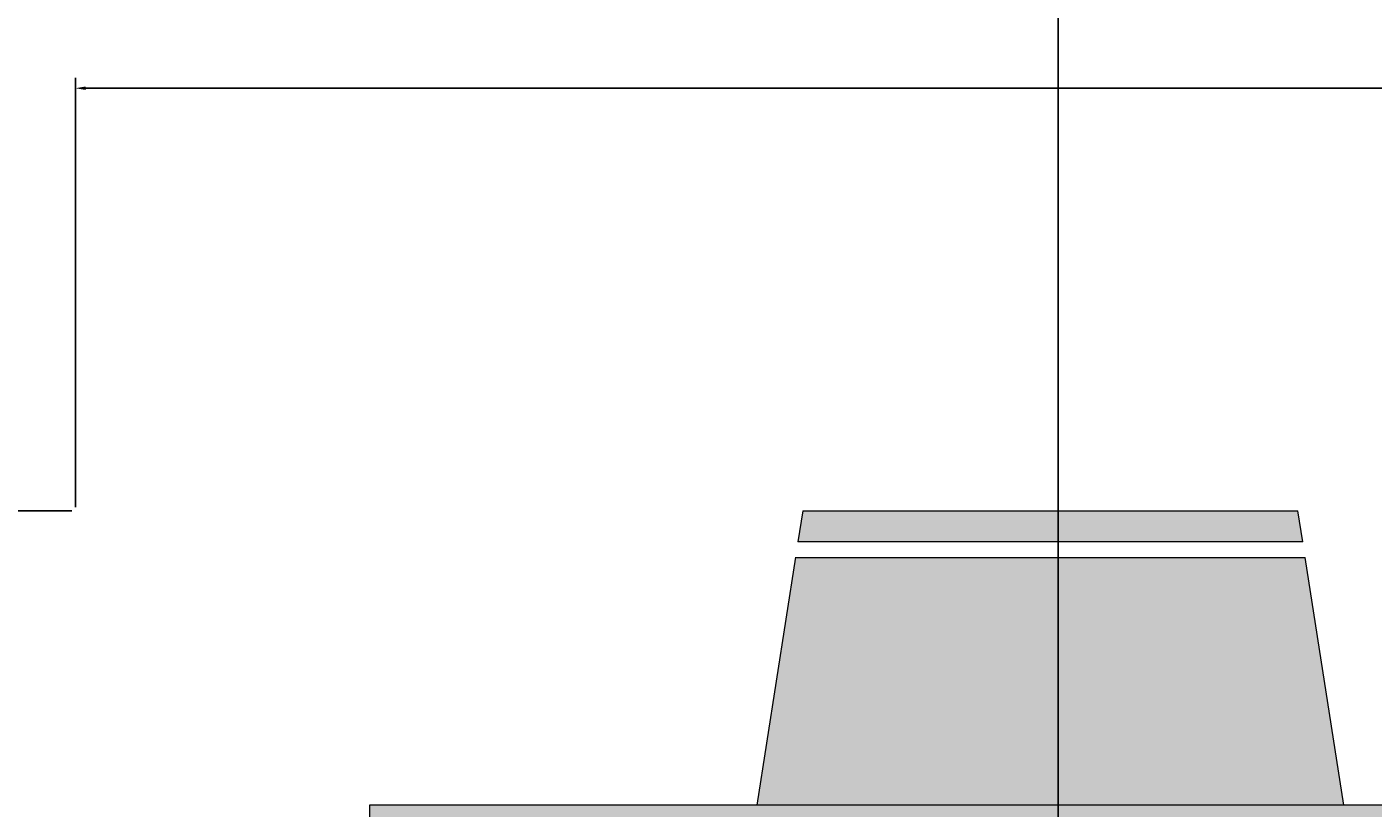
# Model space of a CAD drawing. Units: inches. Extents: x 2549 to 3108, y 1683 to 2362.
# Tile 10 of 30: x 2711 to 2734, y 2041 to 2055. Entities that reach past the tile are written whole.
import ezdxf

# ---------------------------------------------------------------- set-up
doc = ezdxf.new("R2010")
doc.units = ezdxf.units.IN
for name, color, linetype, lineweight in [('A-ANNO-DIMS', 2, 'Continuous', 18), ('A-FURN', 8, 'Continuous', 18), ('A-FURN-PATT', 9, 'Continuous', 13)]:
    doc.layers.add(name, color=color, linetype=linetype, lineweight=lineweight)
doc.layers.add('C-PKNG-VEHI-PATT', color=251, linetype='Continuous', lineweight=13, true_color=0x636466)
doc.layers.add('C-PVMT-PATT', color=9, linetype='Continuous', lineweight=13, true_color=0xc7c8ca)
doc.styles.get("Standard").update_dxf_attribs({"font": 'arial.ttf'})
doc.dimstyles.get("Standard").update_dxf_attribs({"dimtxt": 0.18, "dimasz": 0.18, "dimexe": 0.18, "dimexo": 0.0625, "dimgap": 0.09, "dimtad": 0, "dimtih": 1, "dimtoh": 1, "dimdec": 4, "dimzin": 0, "dimdsep": 46, "dimtxsty": 'Standard', "dimcen": 0.09, "dimadec": 0, "dimazin": 0, "dimtfac": 1, "dimtdec": 4, "dimtofl": 0, "dimtmove": 0, "dimatfit": 3, "dimfxl": 1, "dimtolj": 1, "dimtzin": 0, "dimarcsym": 0})

# ---------------------------------------------------------------- blocks, each defined once
blk = doc.blocks.new('Dining Set - 36 x 72 in.')
for p, q in [((-22, 27.5), (-22.1562, 26.50042)), ((-22, 27.5), (-6, 27.5)), ((-5.8437, 26.49966), (-6, 27.5)), ((-5.8416, 26.5), (-22.1534, 26.5)), ((-22.2343, 26.00059), (-23.4847, 17.99762)), ((-22.2304, 26), (-5.7608, 26)), ((-4.5152, 17.99762), (-5.7655, 25.99926)), ((36, 18), (-36, 18)), ((-36, 18), (-36, -18))]:
    blk.add_line(p, q)
blk = doc.blocks.new('*D20')
at = {"layer": 'A-ANNO-DIMS', "color": 0, "lineweight": -2, "transparency": 16777216}
for p, q in [((2711.514, 2046.346), (2711.514, 2053.826)), ((2711.694, 2053.646), (2735.087, 2053.646)), ((2760.417, 2053.646), (2737.025, 2053.646)), ((2760.597, 2046.346), (2760.597, 2053.826))]:
    blk.add_line(p, q, dxfattribs=at)
at = {"layer": 'A-ANNO-DIMS', "color": 0, "transparency": 16777216}
for points in [[(2711.694, 2053.676), (2711.694, 2053.616), (2711.514, 2053.646)], [(2760.417, 2053.676), (2760.417, 2053.616), (2760.597, 2053.646)]]:
    blk.add_solid(points, dxfattribs=at)
at = {"layer": 'Defpoints', "color": 0, "transparency": 16777216}
for p in [(2760.597, 2053.646), (2711.514, 2046.283), (2760.597, 2046.283)]:
    blk.add_point(p, dxfattribs=at)
at = {"layer": 'A-ANNO-DIMS', "color": 0, "transparency": 16777216, "insert": (2736.056, 2053.646), "char_height": 0.18, "attachment_point": 5}
blk.add_mtext('\\A1;DINING SET 49', dxfattribs=at)
blk = doc.blocks.new('*D21')
at = {"layer": 'A-ANNO-DIMS', "color": 0, "lineweight": -2, "transparency": 16777216}
for p, q in [((2711.452, 2046.283), (2703.972, 2046.283)), ((2704.152, 2046.103), (2704.152, 2031.633)), ((2704.152, 2016.798), (2704.152, 2031.269)), ((2711.452, 2016.618), (2703.972, 2016.618))]:
    blk.add_line(p, q, dxfattribs=at)
at = {"layer": 'A-ANNO-DIMS', "color": 0, "transparency": 16777216}
for points in [[(2704.122, 2046.103), (2704.182, 2046.103), (2704.152, 2046.283)], [(2704.122, 2016.798), (2704.182, 2016.798), (2704.152, 2016.618)]]:
    blk.add_solid(points, dxfattribs=at)
at = {"layer": 'Defpoints', "color": 0, "transparency": 16777216}
for p in [(2704.152, 2046.283), (2711.514, 2046.283), (2711.514, 2016.618)]:
    blk.add_point(p, dxfattribs=at)
at = {"layer": 'A-ANNO-DIMS', "color": 0, "transparency": 16777216, "insert": (2704.152, 2031.451), "char_height": 0.18, "attachment_point": 5}
blk.add_mtext('\\A1;30', dxfattribs=at)
blk = doc.blocks.new('*D42')
at = {"layer": 'A-ANNO-DIMS', "color": 0, "lineweight": -2, "transparency": 16777216}
for p, q in [((2638.643, 2080.461), (2638.643, 1683.444)), ((2728.643, 2080.461), (2728.643, 1683.444)), ((2638.823, 1683.624), (2683.424, 1683.624)), ((2728.463, 1683.624), (2683.861, 1683.624))]:
    blk.add_line(p, q, dxfattribs=at)
at = {"layer": 'A-ANNO-DIMS', "color": 0, "transparency": 16777216}
for points in [[(2638.823, 1683.654), (2638.823, 1683.594), (2638.643, 1683.624)], [(2728.463, 1683.654), (2728.463, 1683.594), (2728.643, 1683.624)]]:
    blk.add_solid(points, dxfattribs=at)
at = {"layer": 'Defpoints', "color": 0, "transparency": 16777216}
for p in [(2638.643, 2080.524), (2728.643, 2080.524), (2728.643, 1683.624)]:
    blk.add_point(p, dxfattribs=at)
at = {"layer": 'A-ANNO-DIMS', "color": 0, "transparency": 16777216, "insert": (2683.643, 1683.624), "char_height": 0.18, "attachment_point": 5}
blk.add_mtext('\\A1;90', dxfattribs=at)
blk = doc.blocks.new('*D59')
at = {"layer": 'A-ANNO-DIMS', "color": 0, "lineweight": -2, "transparency": 16777216}
for p, q in [((2680.978, 1761.586), (2680.978, 2362.323)), ((2681.158, 2362.143), (2733.112, 2362.143)), ((2785.978, 2362.143), (2734.023, 2362.143)), ((2786.158, 1761.586), (2786.158, 2362.323))]:
    blk.add_line(p, q, dxfattribs=at)
at = {"layer": 'A-ANNO-DIMS', "color": 0, "transparency": 16777216}
for points in [[(2681.158, 2362.173), (2681.158, 2362.113), (2680.978, 2362.143)], [(2785.978, 2362.173), (2785.978, 2362.113), (2786.158, 2362.143)]]:
    blk.add_solid(points, dxfattribs=at)
at = {"layer": 'Defpoints', "color": 0, "transparency": 16777216}
for p in [(2786.158, 2362.143), (2680.978, 1761.524), (2786.158, 1761.524)]:
    blk.add_point(p, dxfattribs=at)
at = {"layer": 'A-ANNO-DIMS', "color": 0, "transparency": 16777216, "insert": (2733.568, 2362.143), "char_height": 0.18, "attachment_point": 5}
blk.add_mtext('\\A1;105.18', dxfattribs=at)

msp = doc.modelspace()

# ---------------------------------------------------------------- hatches: boundary and pattern name
at = {"layer": 'A-FURN-PATT'}
h = msp.add_hatch(color=256, dxfattribs=at)
h.dxf.hatch_style = 1
h.paths.add_polyline_path([(2732.9458, 2045.4744), (2724.0631, 2045.4744), (2723.389, 2041.1594), (2733.6201, 2041.1594)])
h.paths.add_polyline_path([(2748.0481, 2045.4744), (2739.1654, 2045.4744), (2738.4912, 2041.1594), (2748.7223, 2041.1594)])
h.paths.add_polyline_path([(2747.9217, 2046.2834), (2739.2918, 2046.2834), (2739.2075, 2045.7441), (2748.006, 2045.7441)])
h.paths.add_polyline_path([(2732.8194, 2046.2834), (2724.1896, 2046.2834), (2724.1053, 2045.7441), (2732.9037, 2045.7441)])
h.paths.add_polyline_path([(2759.7877, 2035.8922), (2755.4728, 2036.5664), (2755.4728, 2026.3353), (2759.7877, 2027.0095)])
h.paths.add_polyline_path([(2760.5968, 2035.7658), (2760.0574, 2035.8501), (2760.0574, 2027.0516), (2760.5968, 2027.1359)])
h.paths.add_polyline_path([(2716.6384, 2036.5664), (2712.3235, 2035.8922), (2712.3235, 2027.0095), (2716.6384, 2026.3353)])
h.paths.add_polyline_path([(2733.6201, 2021.7423), (2723.389, 2021.7423), (2724.0631, 2017.4273), (2732.9458, 2017.4273)])
h.paths.add_polyline_path([(2748.7223, 2021.7423), (2738.4912, 2021.7423), (2739.1654, 2017.4273), (2748.0481, 2017.4273)])
h.paths.add_polyline_path([(2748.006, 2017.1576), (2739.2075, 2017.1576), (2739.2918, 2016.6183), (2747.9217, 2016.6183)])
h.paths.add_polyline_path([(2732.9037, 2017.1576), (2724.1053, 2017.1576), (2724.1896, 2016.6183), (2732.8194, 2016.6183)])
h.paths.add_polyline_path([(2712.0538, 2035.85), (2711.5145, 2035.7658), (2711.5145, 2027.1359), (2712.0538, 2027.0516)])
h = msp.add_hatch(color=256, dxfattribs=at)
h.dxf.hatch_style = 1
h.paths.add_polyline_path([(2744.8667, 2037.254), (2744.7754, 2037.3839), (2744.7125, 2037.4849), (2744.6595, 2037.5854), (2744.5963, 2037.7375), (2744.5695, 2037.9287), (2744.6003, 2038.0617), (2744.6406, 2038.148), (2744.7014, 2038.2298), (2744.7817, 2038.3053), (2744.8799, 2038.3724), (2744.9945, 2038.4289), (2745.1238, 2038.4728), (2745.2663, 2038.5019), (2745.4204, 2038.5142), (2745.5844, 2038.5076), (2745.7585, 2038.4805), (2745.9486, 2038.4342), (2746.1624, 2038.3705), (2746.4075, 2038.2913), (2746.6917, 2038.1983), (2747.0224, 2038.0936), (2747.4074, 2037.9788), (2747.8543, 2037.8558), (2748.3724, 2037.7256), (2748.9783, 2037.5851), (2749.69, 2037.4304), (2750.5258, 2037.2575), (2751.5038, 2037.0624), (2752.6422, 2036.8414), (2753.9591, 2036.5902), (2755.4728, 2036.3051), (2755.4728, 2039.002), (2754.0892, 2039.103), (2752.7721, 2039.2035), (2751.5251, 2039.303), (2750.3516, 2039.4009), (2749.255, 2039.4967), (2748.2388, 2039.5898), (2747.3063, 2039.6798), (2746.4609, 2039.7661), (2745.7045, 2039.8482), (2745.0321, 2039.9255), (2744.4371, 2039.9976), (2743.9129, 2040.0639), (2743.4531, 2040.1238), (2743.0509, 2040.1769), (2742.6998, 2040.2227), (2742.3932, 2040.2605), (2742.1251, 2040.29), (2741.8917, 2040.3111), (2741.69, 2040.3237), (2741.5167, 2040.3279), (2741.3687, 2040.3237), (2741.2428, 2040.3111), (2741.1359, 2040.29), (2741.0448, 2040.2605), (2740.9668, 2040.2227), (2740.9015, 2040.1776), (2740.8488, 2040.1262), (2740.8088, 2040.0695), (2740.7814, 2040.0085), (2740.7667, 2039.9445), (2740.7646, 2039.8783), (2740.7751, 2039.811), (2740.7978, 2039.7435), (2740.8306, 2039.6755), (2740.8707, 2039.6064), (2740.9155, 2039.5357), (2740.996, 2039.4111), (2741.0771, 2039.2637), (2741.1346, 2039.0945), (2741.1499, 2038.9139), (2741.1092, 2038.7391), (2741.0289, 2038.6239), (2740.9549, 2038.5525), (2740.8586, 2038.4895), (2740.733, 2038.4359), (2740.5693, 2038.3929), (2740.3593, 2038.3615), (2740.0946, 2038.3427), (2739.7666, 2038.3376), (2739.367, 2038.3473), (2738.8873, 2038.3727), (2738.3203, 2038.4145), (2737.6635, 2038.471), (2736.9156, 2038.5402), (2736.0753, 2038.6199), (2735.1412, 2038.7081), (2734.112, 2038.8025), (2732.9864, 2038.9012), (2731.7632, 2039.002), (2730.4376, 2039.1026), (2728.9922, 2039.2), (2727.4062, 2039.2911), (2725.6588, 2039.3728), (2723.7291, 2039.4418), (2721.5964, 2039.495), (2719.2397, 2039.5292), (2716.6384, 2039.5413), (2716.6384, 2036.8445), (2720.4266, 2036.9215), (2723.5572, 2036.9548), (2726.1183, 2036.9512), (2728.1983, 2036.9175), (2729.8853, 2036.8608), (2731.2677, 2036.7876), (2732.4336, 2036.705), (2733.4711, 2036.6198), (2734.4538, 2036.5375), (2735.3951, 2036.4589), (2736.2938, 2036.3835), (2737.1484, 2036.3108), (2737.9578, 2036.2401), (2738.7205, 2036.171), (2739.4353, 2036.103), (2740.1009, 2036.0355), (2740.7163, 2035.9683), (2741.2828, 2035.9027), (2741.8019, 2035.8403), (2742.2752, 2035.7826), (2742.7042, 2035.7313), (2743.0906, 2035.6878), (2743.4358, 2035.6539), (2743.7416, 2035.6309), (2744.0097, 2035.6203), (2744.243, 2035.6218), (2744.4448, 2035.6349), (2744.6181, 2035.659), (2744.7661, 2035.6937), (2744.892, 2035.7384), (2744.9989, 2035.7926), (2745.09, 2035.8557), (2745.1679, 2035.9271), (2745.2326, 2036.006), (2745.2836, 2036.0911), (2745.3204, 2036.1815), (2745.3424, 2036.2762), (2745.3492, 2036.374), (2745.3401, 2036.4739), (2745.3148, 2036.5748), (2745.2731, 2036.676), (2745.2178, 2036.7771), (2745.152, 2036.8782), (2745.0788, 2036.9794), (2745.0013, 2037.0805)])
h.paths.add_polyline_path([(2755.4728, 2036.3051), (2753.9591, 2036.5902), (2752.6422, 2036.8414), (2751.5038, 2037.0624), (2750.5258, 2037.2575), (2749.69, 2037.4304), (2748.9783, 2037.5851), (2748.3724, 2037.7256), (2747.8543, 2037.8558), (2747.4074, 2037.9788), (2747.0224, 2038.0936), (2746.6917, 2038.1983), (2746.4075, 2038.2913), (2746.1624, 2038.3705), (2745.9486, 2038.4342), (2745.7585, 2038.4805), (2745.5844, 2038.5076), (2745.4204, 2038.5142), (2745.2663, 2038.5019), (2745.1238, 2038.4728), (2744.9945, 2038.4289), (2744.8799, 2038.3724), (2744.7817, 2038.3053), (2744.7014, 2038.2298), (2744.6406, 2038.148), (2744.6003, 2038.0617), (2744.5794, 2037.9717), (2744.5765, 2037.8786), (2744.59, 2037.7828), (2744.6182, 2037.6849), (2744.6595, 2037.5854), (2744.7125, 2037.4849), (2744.7754, 2037.3839), (2744.8465, 2037.2827), (2744.9229, 2037.1816), (2745.0013, 2037.0805), (2745.1278, 2036.9154), (2745.2178, 2036.7771), (2745.2731, 2036.676), (2745.3148, 2036.5748), (2745.3401, 2036.4739), (2745.3492, 2036.374), (2745.3424, 2036.2762), (2745.3204, 2036.1815), (2745.2836, 2036.0911), (2745.2326, 2036.006), (2745.1679, 2035.9271), (2745.09, 2035.8557), (2744.9989, 2035.7926), (2744.892, 2035.7384), (2744.7661, 2035.6937), (2744.6181, 2035.659), (2744.4448, 2035.6349), (2744.243, 2035.6218), (2744.0097, 2035.6203), (2743.7416, 2035.6309), (2743.4358, 2035.6539), (2743.0906, 2035.6878), (2742.7042, 2035.7313), (2742.2752, 2035.7826), (2741.8019, 2035.8403), (2741.2828, 2035.9027), (2740.7163, 2035.9683), (2740.1009, 2036.0355), (2739.4353, 2036.103), (2738.7205, 2036.171), (2737.9578, 2036.2401), (2737.1484, 2036.3108), (2736.2938, 2036.3835), (2735.3951, 2036.4589), (2734.4538, 2036.5375), (2733.4711, 2036.6198), (2732.4336, 2036.705), (2731.2677, 2036.7876), (2729.8853, 2036.8608), (2728.1983, 2036.9175), (2726.1183, 2036.9512), (2723.5572, 2036.9548), (2720.4266, 2036.9215), (2716.6384, 2036.8445), (2716.6384, 2034.4174), (2719.4886, 2034.3283), (2721.9949, 2034.2608), (2724.1925, 2034.2112), (2726.1167, 2034.1758), (2727.8028, 2034.1509), (2729.2861, 2034.1329), (2730.602, 2034.1181), (2731.7856, 2034.1027), (2732.8685, 2034.0839), (2733.8666, 2034.0613), (2734.7919, 2034.0356), (2735.6567, 2034.0072), (2736.473, 2033.9768), (2737.253, 2033.9447), (2738.0088, 2033.9116), (2738.7525, 2033.878), (2739.493, 2033.8445), (2740.2273, 2033.812), (2740.9489, 2033.7816), (2741.6515, 2033.7544), (2742.3289, 2033.7314), (2742.9747, 2033.7137), (2743.5825, 2033.7022), (2744.1461, 2033.6982), (2744.6607, 2033.7024), (2745.1272, 2033.7151), (2745.5485, 2033.7361), (2745.9272, 2033.7656), (2746.2658, 2033.8036), (2746.567, 2033.8499), (2746.8334, 2033.9047), (2747.0677, 2033.9679), (2747.2728, 2034.0393), (2747.4525, 2034.1175), (2747.6113, 2034.201), (2747.7531, 2034.2881), (2747.8824, 2034.3774), (2748.0032, 2034.4672), (2748.1197, 2034.556), (2748.2363, 2034.6421), (2748.3567, 2034.7241), (2748.4828, 2034.8008), (2748.6163, 2034.8712), (2748.7588, 2034.9343), (2748.9118, 2034.9889), (2749.077, 2035.034), (2749.2558, 2035.0686), (2749.4499, 2035.0916), (2749.6603, 2035.1022), (2749.8861, 2035.1007), (2750.1254, 2035.0876), (2750.3769, 2035.0635), (2750.639, 2035.0288), (2750.91, 2034.9841), (2751.1884, 2034.93), (2751.4725, 2034.8668), (2751.7642, 2034.7949), (2752.0786, 2034.7123), (2752.4341, 2034.6172), (2752.849, 2034.5073), (2753.3419, 2034.3805), (2753.9313, 2034.2348), (2754.6354, 2034.068), (2755.4728, 2033.878)])
h.paths.add_polyline_path([(2755.4728, 2033.878), (2754.6354, 2034.068), (2753.9313, 2034.2348), (2753.3419, 2034.3805), (2752.849, 2034.5073), (2752.4341, 2034.6172), (2752.0786, 2034.7123), (2751.7642, 2034.7949), (2751.4725, 2034.8668), (2751.1884, 2034.93), (2750.91, 2034.9841), (2750.639, 2035.0288), (2750.3769, 2035.0635), (2750.1254, 2035.0876), (2749.8861, 2035.1007), (2749.6603, 2035.1022), (2749.4499, 2035.0916), (2749.2558, 2035.0686), (2749.077, 2035.034), (2748.9118, 2034.9889), (2748.7588, 2034.9343), (2748.6163, 2034.8712), (2748.4828, 2034.8008), (2748.3567, 2034.7241), (2748.2363, 2034.6421), (2748.1197, 2034.556), (2748.0032, 2034.4672), (2747.8824, 2034.3774), (2747.7531, 2034.2881), (2747.6113, 2034.201), (2747.4525, 2034.1175), (2747.2728, 2034.0393), (2747.0677, 2033.9679), (2746.8334, 2033.9047), (2746.567, 2033.8499), (2746.2658, 2033.8036), (2745.9272, 2033.7656), (2745.5485, 2033.7361), (2745.1272, 2033.7151), (2744.6607, 2033.7024), (2744.1461, 2033.6982), (2743.5825, 2033.7022), (2742.9747, 2033.7137), (2742.3289, 2033.7314), (2741.6515, 2033.7544), (2740.9489, 2033.7816), (2740.2273, 2033.812), (2739.493, 2033.8445), (2738.7525, 2033.878), (2738.0088, 2033.9116), (2737.253, 2033.9447), (2736.473, 2033.9768), (2735.6567, 2034.0072), (2734.7919, 2034.0356), (2733.8666, 2034.0613), (2732.8685, 2034.0839), (2731.7856, 2034.1027), (2730.602, 2034.1181), (2729.2861, 2034.1329), (2727.8028, 2034.1509), (2726.1167, 2034.1758), (2724.1925, 2034.2112), (2721.9949, 2034.2608), (2719.4886, 2034.3283), (2716.6384, 2034.4174), (2716.6384, 2030.9115), (2719.4477, 2031.0954), (2722.0216, 2031.2447), (2724.3773, 2031.363), (2726.5324, 2031.4537), (2728.5042, 2031.5201), (2730.3101, 2031.5657), (2731.9674, 2031.5939), (2733.4936, 2031.6082), (2734.9046, 2031.6115), (2736.2109, 2031.6057), (2737.4211, 2031.592), (2738.5446, 2031.5716), (2739.59, 2031.5461), (2740.5665, 2031.5165), (2741.4829, 2031.4843), (2742.3482, 2031.4509), (2743.1698, 2031.4174), (2743.9488, 2031.3855), (2744.6845, 2031.3568), (2745.3766, 2031.3329), (2746.0244, 2031.3152), (2746.6274, 2031.3055), (2747.1851, 2031.3052), (2747.697, 2031.316), (2748.1634, 2031.3388), (2748.5882, 2031.3722), (2748.9761, 2031.414), (2749.3319, 2031.4621), (2749.6603, 2031.5144), (2749.9661, 2031.5688), (2750.254, 2031.6233), (2750.5287, 2031.6756), (2750.7946, 2031.7239), (2751.0553, 2031.7669), (2751.314, 2031.8036), (2751.5737, 2031.8329), (2751.8375, 2031.8538), (2752.1088, 2031.8652), (2752.3906, 2031.8661), (2752.6861, 2031.8554), (2752.9965, 2031.8326), (2753.315, 2031.7999), (2753.633, 2031.7598), (2753.9418, 2031.7149), (2754.2327, 2031.6679), (2754.497, 2031.6215), (2754.7259, 2031.5782), (2754.911, 2031.5407), (2755.0467, 2031.5111), (2755.141, 2031.4888), (2755.2053, 2031.4728), (2755.2509, 2031.4621), (2755.2891, 2031.4556), (2755.3313, 2031.4523), (2755.3888, 2031.451), (2755.4728, 2031.4509)])
h.paths.add_polyline_path([(2743.9488, 2031.3855), (2743.1698, 2031.4174), (2742.3482, 2031.4509), (2741.4829, 2031.4843), (2740.5665, 2031.5165), (2739.59, 2031.5461), (2738.5446, 2031.5716), (2737.4211, 2031.592), (2736.2109, 2031.6057), (2734.9046, 2031.6115), (2733.4936, 2031.6082), (2731.9674, 2031.5939), (2730.3101, 2031.5657), (2728.5042, 2031.5201), (2726.5324, 2031.4537), (2724.3773, 2031.363), (2722.0216, 2031.2447), (2719.4477, 2031.0954), (2716.6384, 2030.9115), (2716.6384, 2027.945), (2721.3933, 2028.046), (2725.223, 2028.1465), (2728.2515, 2028.246), (2730.603, 2028.3439), (2732.4013, 2028.4397), (2733.7707, 2028.5328), (2734.8351, 2028.6228), (2735.7185, 2028.7091), (2736.5253, 2028.7912), (2737.2808, 2028.8692), (2737.9904, 2028.9429), (2738.6597, 2029.0125), (2739.2943, 2029.0778), (2739.8997, 2029.1389), (2740.4813, 2029.1958), (2741.0448, 2029.2484), (2741.5952, 2029.2967), (2742.1361, 2029.3397), (2742.6708, 2029.3764), (2743.2022, 2029.4058), (2743.7337, 2029.4266), (2744.2683, 2029.4381), (2744.8093, 2029.4389), (2745.3597, 2029.4282), (2745.9213, 2029.4053), (2746.4897, 2029.3713), (2747.0592, 2029.3279), (2747.6239, 2029.2765), (2748.1781, 2029.2189), (2748.716, 2029.1564), (2749.2317, 2029.0909), (2749.7196, 2029.0237), (2750.1754, 2028.9563), (2750.602, 2028.8892), (2751.0039, 2028.8226), (2751.3854, 2028.7568), (2751.7512, 2028.6921), (2752.1057, 2028.6287), (2752.4532, 2028.5668), (2752.7985, 2028.5068), (2753.1447, 2028.4496), (2753.4913, 2028.399), (2753.8363, 2028.3595), (2754.1778, 2028.3355), (2754.514, 2028.3315), (2754.8432, 2028.352), (2755.1634, 2028.4014), (2755.4728, 2028.4843), (2755.4728, 2031.4509), (2755.3151, 2031.4512), (2755.2429, 2031.4634), (2755.141, 2031.4888), (2755.0467, 2031.5111), (2754.911, 2031.5407), (2754.7259, 2031.5782), (2754.497, 2031.6215), (2754.2327, 2031.6679), (2753.9418, 2031.7149), (2753.633, 2031.7598), (2753.315, 2031.7999), (2752.9965, 2031.8326), (2752.6861, 2031.8554), (2752.3906, 2031.8661), (2752.1088, 2031.8652), (2751.8375, 2031.8538), (2751.5737, 2031.8329), (2751.314, 2031.8036), (2751.0553, 2031.7669), (2750.7946, 2031.7239), (2750.5287, 2031.6756), (2750.254, 2031.6233), (2749.9661, 2031.5688), (2749.6603, 2031.5144), (2749.3319, 2031.4621), (2748.9761, 2031.414), (2748.5882, 2031.3722), (2748.1634, 2031.3388), (2747.697, 2031.316), (2747.1851, 2031.3052), (2746.6274, 2031.3055), (2746.0244, 2031.3152), (2745.3766, 2031.3329), (2744.6845, 2031.3568)])
h.paths.add_polyline_path([(2755.4728, 2028.4843), (2755.1634, 2028.4014), (2754.8432, 2028.352), (2754.514, 2028.3315), (2754.1778, 2028.3355), (2753.8363, 2028.3595), (2753.4913, 2028.399), (2753.1447, 2028.4496), (2752.7985, 2028.5068), (2752.4532, 2028.5668), (2752.1057, 2028.6287), (2751.7512, 2028.6921), (2751.3854, 2028.7568), (2751.0039, 2028.8226), (2750.602, 2028.8892), (2750.1754, 2028.9563), (2749.7196, 2029.0237), (2749.2317, 2029.0909), (2748.716, 2029.1564), (2748.1781, 2029.2189), (2747.6239, 2029.2765), (2747.0592, 2029.3279), (2746.4897, 2029.3713), (2745.9213, 2029.4053), (2745.3597, 2029.4282), (2744.8093, 2029.4389), (2744.2683, 2029.4381), (2743.7337, 2029.4266), (2743.2022, 2029.4058), (2742.6708, 2029.3764), (2742.1361, 2029.3397), (2741.5952, 2029.2967), (2741.0448, 2029.2484), (2740.4813, 2029.1958), (2739.8997, 2029.1389), (2739.2943, 2029.0778), (2738.6597, 2029.0125), (2737.9904, 2028.9429), (2737.2808, 2028.8692), (2736.5253, 2028.7912), (2735.7185, 2028.7091), (2734.8351, 2028.6228), (2733.7707, 2028.5328), (2732.4013, 2028.4397), (2730.603, 2028.3439), (2728.2515, 2028.246), (2725.223, 2028.1465), (2721.3933, 2028.046), (2716.6384, 2027.945), (2716.6384, 2023.63), (2719.8271, 2023.719), (2722.5536, 2023.7853), (2724.8739, 2023.8315), (2726.8443, 2023.8604), (2728.5207, 2023.8745), (2729.9593, 2023.8765), (2731.2162, 2023.8691), (2732.3475, 2023.8548), (2733.4006, 2023.8359), (2734.3887, 2023.8133), (2735.3162, 2023.7876), (2736.1877, 2023.7593), (2737.0074, 2023.7288), (2737.7801, 2023.6968), (2738.5101, 2023.6637), (2739.2019, 2023.63), (2739.8611, 2023.5965), (2740.4973, 2023.5644), (2741.1215, 2023.5348), (2741.7443, 2023.5092), (2742.3766, 2023.4889), (2743.0291, 2023.4752), (2743.7127, 2023.4693), (2744.4383, 2023.4727), (2745.2212, 2023.4875), (2746.096, 2023.5194), (2747.1021, 2023.575), (2748.2785, 2023.6609), (2749.6645, 2023.7837), (2751.2994, 2023.9499), (2753.2224, 2024.1662), (2755.4728, 2024.4391)])
h.paths.add_polyline_path([(2755.4728, 2026.3269), (2754.9554, 2026.3329), (2754.418, 2026.3497), (2753.8658, 2026.3755), (2753.3041, 2026.4083), (2752.7382, 2026.4465), (2752.1734, 2026.4881), (2751.6149, 2026.5312), (2751.068, 2026.5741), (2750.5357, 2026.6151), (2750.0124, 2026.6538), (2749.4902, 2026.6898), (2748.9611, 2026.723), (2748.4173, 2026.753), (2747.8508, 2026.7795), (2747.2537, 2026.8024), (2746.6182, 2026.8213), (2745.9367, 2026.8359), (2745.2024, 2026.8452), (2744.4091, 2026.8482), (2743.5505, 2026.8438), (2742.6204, 2026.8309), (2741.6122, 2026.8087), (2740.5198, 2026.7758), (2739.3368, 2026.7314), (2738.0388, 2026.6748), (2736.5297, 2026.6071), (2734.695, 2026.5299), (2732.4205, 2026.4449), (2729.5919, 2026.3535), (2726.0949, 2026.2573), (2721.8152, 2026.1581), (2716.6384, 2026.0572), (2716.6384, 2023.63), (2719.8271, 2023.719), (2722.5536, 2023.7853), (2724.8739, 2023.8315), (2726.8443, 2023.8604), (2728.5207, 2023.8745), (2729.9593, 2023.8765), (2731.2162, 2023.8691), (2732.3475, 2023.8548), (2733.4006, 2023.8359), (2734.3887, 2023.8133), (2735.3162, 2023.7876), (2736.1877, 2023.7593), (2737.0074, 2023.7288), (2737.7801, 2023.6968), (2738.5101, 2023.6637), (2739.2019, 2023.63), (2739.8611, 2023.5965), (2740.4973, 2023.5644), (2741.1215, 2023.5348), (2741.7443, 2023.5092), (2742.3766, 2023.4889), (2743.0291, 2023.4752), (2743.7127, 2023.4693), (2744.4383, 2023.4727), (2745.2212, 2023.4875), (2746.096, 2023.5194), (2747.1021, 2023.575), (2748.2785, 2023.6609), (2749.6645, 2023.7837), (2751.2994, 2023.9499), (2753.2224, 2024.1662), (2755.4728, 2024.4391)], flags=17)
h.paths.add_polyline_path([(2740.4973, 2023.5644), (2739.8611, 2023.5965), (2739.2019, 2023.63), (2738.5101, 2023.6637), (2737.7801, 2023.6968), (2737.0074, 2023.7288), (2736.1877, 2023.7593), (2735.3162, 2023.7876), (2734.3887, 2023.8133), (2733.4006, 2023.8359), (2732.3475, 2023.8548), (2731.2162, 2023.8691), (2729.9593, 2023.8765), (2728.5207, 2023.8745), (2726.8443, 2023.8604), (2724.8739, 2023.8315), (2722.5536, 2023.7853), (2719.8271, 2023.719), (2716.6384, 2023.63), (2716.6384, 2021.7423), (2755.4728, 2021.7423), (2755.4728, 2024.4391), (2753.2224, 2024.1662), (2751.2994, 2023.9499), (2749.6645, 2023.7837), (2748.2785, 2023.6609), (2747.1021, 2023.575), (2746.096, 2023.5194), (2745.2212, 2023.4875), (2744.4383, 2023.4727), (2743.7127, 2023.4693), (2743.0291, 2023.4752), (2742.3766, 2023.4889), (2741.7443, 2023.5092), (2741.1215, 2023.5348)])
h.paths.add_polyline_path([(2741.1359, 2040.29), (2741.2428, 2040.3111), (2741.3687, 2040.3237), (2741.5167, 2040.3279), (2741.69, 2040.3237), (2741.8917, 2040.3111), (2742.1251, 2040.29), (2742.3932, 2040.2605), (2742.6998, 2040.2227), (2743.0509, 2040.1769), (2743.4531, 2040.1238), (2743.9129, 2040.0639), (2744.4371, 2039.9976), (2745.0321, 2039.9255), (2745.7045, 2039.8482), (2746.4609, 2039.7661), (2747.3063, 2039.6798), (2748.2388, 2039.5898), (2749.255, 2039.4967), (2750.3516, 2039.4009), (2751.5251, 2039.303), (2752.7721, 2039.2035), (2754.0892, 2039.103), (2755.4728, 2039.002), (2755.4728, 2041.1594), (2716.6384, 2041.1594), (2716.6384, 2039.5413), (2719.2397, 2039.5292), (2721.5964, 2039.495), (2723.7291, 2039.4418), (2725.6588, 2039.3728), (2727.4062, 2039.2911), (2728.9922, 2039.2), (2730.4376, 2039.1026), (2731.7632, 2039.002), (2732.9864, 2038.9012), (2734.112, 2038.8025), (2735.1412, 2038.7081), (2736.0753, 2038.6199), (2736.9156, 2038.5402), (2737.6635, 2038.471), (2738.3203, 2038.4145), (2738.8873, 2038.3727), (2739.367, 2038.3473), (2739.7666, 2038.3376), (2740.0946, 2038.3427), (2740.3593, 2038.3615), (2740.5693, 2038.3929), (2740.733, 2038.4359), (2740.8586, 2038.4895), (2740.9549, 2038.5525), (2741.0289, 2038.6239), (2741.0834, 2038.7021), (2741.12, 2038.7856), (2741.1403, 2038.8728), (2741.1458, 2038.962), (2741.1382, 2039.0518), (2741.1189, 2039.1406), (2741.0897, 2039.2267), (2741.0522, 2039.309), (2741.0089, 2039.3875), (2740.9625, 2039.4629), (2740.8772, 2039.5951), (2740.8072, 2039.7159), (2740.7635, 2039.8453), (2740.7677, 2039.9782), (2740.8229, 2040.1009), (2740.9289, 2040.2044), (2741.0448, 2040.2605)])
at = {"layer": 'C-PKNG-VEHI-PATT'}
h = msp.add_hatch(color=256, dxfattribs=at)
h.dxf.hatch_style = 1
edge = h.paths.add_edge_path()
edge.add_ellipse((2935.7258, 1791.964), major_axis=(-50.66, 0), ratio=0.8423039, start_angle=248.16505, end_angle=265.72258)
edge.add_line((2938.911, 1834.5507), (2925.8653, 1834.5507))
edge.add_ellipse((2929.0505, 1791.964), major_axis=(50.66, 0), ratio=0.8423039, start_angle=94.27742, end_angle=111.83495)
edge.add_line((2912.8508, 1832.3947), (2914.2044, 1822.2495))
edge.add_ellipse((2930.6538, 1783.1023), major_axis=(-49.3014, 0), ratio=0.8423039, start_angle=-85.12993, end_angle=-67.20809, ccw=False)
edge.add_line((2927.1247, 1824.5225), (2937.6516, 1824.5225))
edge.add_ellipse((2934.1225, 1783.1023), major_axis=(49.3014, 0), ratio=0.8423039, start_angle=67.20809, end_angle=85.12993, ccw=False)
edge.add_line((2950.5719, 1822.2495), (2951.9255, 1832.3947))
edge = h.paths.add_edge_path()
edge.add_ellipse((2903.4793, 1857.3351), major_axis=(-34.7979, 0), ratio=0.8423039, start_angle=180, end_angle=209.43857)
edge.add_ellipse((2961.297, 1857.3351), major_axis=(34.7979, 0), ratio=0.8423039, start_angle=150.56143, end_angle=180)
edge.add_line((2926.4991, 1857.3351), (2926.4991, 1843.7609))
edge.add_ellipse((2924.1251, 1844.3143), major_axis=(-0.2209, 3.9278), ratio=0.6038336, start_angle=89.00201, end_angle=253.65741, ccw=False)
edge.add_line((2921.7512, 1844.2222), (2921.7512, 1853.3975))
edge.add_line((2921.7512, 1853.3975), (2925.269, 1855.8484))
edge.add_ellipse((2925.4782, 1855.4931), major_axis=(0.4584, 0), ratio=0.8423039, start_angle=90, end_angle=134.48021, ccw=False)
edge.add_line((2925.4782, 1855.8792), (2926.4991, 1855.8792))
edge.add_line((2926.4991, 1855.8792), (2926.4991, 1857.3351))
edge.add_ellipse((2961.297, 1857.3351), major_axis=(34.7979, 0), ratio=0.8423039, start_angle=150.56143, end_angle=180, ccw=False)
edge.add_line((2932.3882, 1873.6501), (2932.3882, 1875.7801))
edge.add_ellipse((2932.3882, 1875.3939), major_axis=(0.4584, 0), ratio=0.8423039, start_angle=90, end_angle=127.93313)
edge.add_line((2932.1366, 1875.7167), (2928.5915, 1873.7564))
edge.add_ellipse((2899.9271, 2002.4692), major_axis=(155.4756, 0), ratio=0.84230387, start_angle=-80.743434, end_angle=-77.445067, ccw=False)
edge.add_ellipse((2949.4402, 1715.2151), major_axis=(-189.1422, 0), ratio=0.84230387, start_angle=-79.790461, end_angle=-77.555373)
edge.add_ellipse((3300.3614, 1852.5642), major_axis=(-386.1662, 0), ratio=0.84230387, start_angle=-2.863715, end_angle=2.198541)
edge.add_ellipse((2929.0505, 1792.5159), major_axis=(-55.6192, 0), ratio=0.8423039, start_angle=-85.91759, end_angle=-72.28005, ccw=False)
edge.add_line((2925.7129, 1839.2798), (2939.0634, 1839.2798))
edge.add_ellipse((2935.7258, 1792.5159), major_axis=(55.6192, 0), ratio=0.8423039, start_angle=72.28005, end_angle=85.91759, ccw=False)
edge.add_ellipse((2564.4149, 1852.5642), major_axis=(-386.1662, 0), ratio=0.84230387, start_angle=177.801459, end_angle=182.863715)
edge.add_ellipse((2915.3361, 1715.2151), major_axis=(189.1422, 0), ratio=0.84230387, start_angle=77.555373, end_angle=79.790461)
edge.add_ellipse((2964.8492, 2002.4692), major_axis=(-155.4756, 0), ratio=0.84230387, start_angle=77.445067, end_angle=80.743434, ccw=False)
edge.add_line((2936.1848, 1873.7564), (2932.6397, 1875.7167))
edge.add_ellipse((2932.3882, 1875.3939), major_axis=(0.4584, 0), ratio=0.8423039, start_angle=52.06687, end_angle=90)
edge.add_line((2932.3882, 1875.7801), (2932.3882, 1873.6501))
edge.add_ellipse((2903.4793, 1857.3351), major_axis=(-34.7979, 0), ratio=0.8423039, start_angle=180, end_angle=209.43857, ccw=False)
edge.add_line((2938.2772, 1857.3351), (2938.2772, 1855.8792))
edge.add_line((2938.2772, 1855.8792), (2939.4059, 1855.8792))
edge.add_ellipse((2939.2981, 1855.4931), major_axis=(-0.4584, 0), ratio=0.8423039, start_angle=225.51979, end_angle=270, ccw=False)
edge.add_line((2939.5903, 1855.7906), (2943.0251, 1853.3975))
edge.add_line((2943.0251, 1853.3975), (2943.0251, 1844.2222))
edge.add_ellipse((2940.6512, 1844.3143), major_axis=(0.2209, 3.9278), ratio=0.6038336, start_angle=106.34259, end_angle=270.99799, ccw=False)
edge.add_line((2938.2772, 1843.7609), (2938.2772, 1857.3351))
edge = h.paths.add_edge_path()
edge.add_ellipse((2932.3882, 1865.1973), major_axis=(91.081, 0), ratio=0.8423039, start_angle=256.401865, end_angle=283.598135, ccw=False)
edge.add_line((2914.2044, 1790.0239), (2914.2044, 1778.3622))
edge.add_ellipse((2932.3882, 1853.5356), major_axis=(91.081, 0), ratio=0.8423039, start_angle=256.401865, end_angle=283.598135)
edge.add_line((2950.5719, 1778.3622), (2950.5719, 1790.0239))
edge = h.paths.add_edge_path()
edge.add_ellipse((2948.7383, 1772.3145), major_axis=(1.8336, 0), ratio=0.8423039, start_angle=0, end_angle=90)
edge.add_line((2948.7383, 1773.859), (2916.038, 1773.859))
edge.add_ellipse((2916.038, 1772.3145), major_axis=(1.8336, 0), ratio=0.8423039, start_angle=90, end_angle=180)
edge.add_line((2914.2044, 1772.3145), (2914.2044, 1760.2558))
edge.add_line((2914.2044, 1760.2558), (2950.5719, 1760.2558))
edge.add_line((2950.5719, 1760.2558), (2950.5719, 1772.3145))
h.paths.add_polyline_path([(2748.8496, 2101.6383), (2798.148, 2101.6383), (2798.148, 2111.4248), (2748.8496, 2111.4248)], flags=9)
h.paths.add_polyline_path([(2685.2081, 2101.489), (2719.3253, 2101.489), (2719.3253, 2111.2819), (2685.2081, 2111.2819)], flags=9)
h.paths.add_polyline_path([(2814.6852, 1907.1328), (2847.8384, 1907.1328), (2847.8384, 1916.9258), (2814.6852, 1916.9258)], flags=9)
h.paths.add_polyline_path([(2814.3906, 1835.5864), (2848.0172, 1835.5864), (2848.0172, 1845.3794), (2814.3906, 1845.3794)], flags=9)
h.paths.add_polyline_path([(2800.5245, 1759.1674), (2853.7435, 1759.1674), (2853.7435, 1768.954), (2800.5245, 1768.954)], flags=9)
h.paths.add_polyline_path([(2972.4611, 1807.3305), (3015.3943, 1807.3305), (3015.3943, 1817.117), (2972.4611, 1817.117)], flags=9)
h.paths.add_polyline_path([(2902.3327, 1888.6731), (2937.9131, 1888.6731), (2937.9131, 1898.4661), (2902.3327, 1898.4661)], flags=9)
h.paths.add_polyline_path([(2712.1779, 1878.9039), (2754.1257, 1878.9039), (2754.1257, 1888.6904), (2712.1779, 1888.6904)], flags=9)
h.paths.add_polyline_path([(2614.0056, 2012.812), (2650.0251, 2012.812), (2650.0251, 2022.4371), (2614.0056, 2022.4371)], flags=9)
h.paths.add_polyline_path([(2713.3129, 2003.1645), (2747.4237, 2003.1645), (2747.4237, 2012.951), (2713.3129, 2012.951)], flags=9)
h.paths.add_polyline_path([(2950.1379, 2001.6934), (2982.2992, 2001.6934), (2982.2992, 2011.48), (2950.1379, 2011.48)], flags=9)
h.paths.add_polyline_path([(2940.864, 2238.5537), (2997.5066, 2238.5537), (2997.5066, 2248.3466), (2940.864, 2248.3466)], flags=9)
h.paths.add_polyline_path([(2821.5457, 2202.8348), (2855.663, 2202.8348), (2855.663, 2212.6278), (2821.5457, 2212.6278)], flags=9)
h.paths.add_polyline_path([(2661.8026, 2238.6249), (2718.4451, 2238.6249), (2718.4451, 2248.4179), (2661.8026, 2248.4179)], flags=9)
at = {"layer": 'C-PVMT-PATT'}
h = msp.add_hatch(color=256, dxfattribs=at)
h.dxf.hatch_style = 1
h.paths.add_polyline_path([(3067.6427, 2305.5237), (2605.6427, 2305.5237), (2605.6427, 2074.5237), (2629.6427, 2074.5237), (2629.6427, 2281.5237), (3043.6427, 2281.5237), (3043.6427, 1885.5237), (3043.6427, 1872.8745), (3031.1672, 1872.8745), (3031.1672, 1862.5731), (2995.8054, 1862.5731), (2995.8054, 1872.8745), (2983.1752, 1872.8745), (2983.1752, 1885.5237), (2881.6427, 1885.5237), (2881.6427, 1795.5237), (2751.0977, 1795.5237), (2751.0977, 1761.5237), (2786.1577, 1761.5237), (2786.1577, 1723.5237), (2881.84, 1723.5237), (2881.84, 1714.5237), (3067.6427, 1714.5237), (3067.6427, 1723.5237)])
edge = h.paths.add_edge_path(flags=16)
edge.add_ellipse((2949.4402, 1710.9683), major_axis=(-194.1014, 0), ratio=0.84230387, start_angle=-77.874034, end_angle=-76.219471, ccw=False)
edge.add_ellipse((2949.4402, 1715.2151), major_axis=(-189.1422, 0), ratio=0.84230387, start_angle=-79.790461, end_angle=-77.555373, ccw=False)
edge.add_ellipse((2899.9271, 2002.4692), major_axis=(155.4756, 0), ratio=0.84230387, start_angle=-80.743434, end_angle=-77.445067)
edge.add_line((2928.5915, 1873.7564), (2932.3882, 1875.8558))
edge.add_line((2932.3882, 1875.8558), (2936.1848, 1873.7564))
edge.add_ellipse((2964.8492, 2002.4692), major_axis=(-155.4756, 0), ratio=0.84230387, start_angle=77.445067, end_angle=80.743434)
edge.add_ellipse((2915.3361, 1715.2151), major_axis=(189.1422, 0), ratio=0.84230387, start_angle=77.555373, end_angle=79.790461, ccw=False)
edge.add_ellipse((2915.3361, 1710.9683), major_axis=(-194.1014, 0), ratio=0.84230387, start_angle=256.219471, end_angle=257.874034, ccw=False)
edge.add_ellipse((2628.2871, 1850.2612), major_axis=(-327.2532, 0), ratio=0.84230387, start_angle=182.17995, end_angle=183.650428, ccw=False)
edge.add_ellipse((2955.5637, 1861.9334), major_axis=(-0.9168, 0), ratio=0.8423039, start_angle=180, end_angle=270, ccw=False)
edge.add_line((2956.4805, 1862.3857), (2956.4805, 1846.4866))
edge.add_ellipse((2955.5637, 1846.939), major_axis=(-0.9168, 0), ratio=0.8423039, start_angle=90, end_angle=180, ccw=False)
edge.add_ellipse((-3607.0606, 1835.832), major_axis=(-6562.6242, 0), ratio=0.84230387, start_angle=179.61613322, end_angle=180.09022909, ccw=False)
edge.add_ellipse((2955.5637, 1791.0926), major_axis=(0.9168, 0), ratio=0.8423039, start_angle=0, end_angle=90, ccw=False)
edge.add_line((2956.4805, 1791.545), (2956.4805, 1775.6459))
edge.add_ellipse((2955.5637, 1776.0982), major_axis=(0.9168, 0), ratio=0.8423039, start_angle=270, end_angle=360, ccw=False)
edge.add_ellipse((-3607.0606, 1835.832), major_axis=(-6562.6242, 0), ratio=0.84230387, start_angle=179.3813568, end_angle=179.47172853, ccw=False)
edge.add_ellipse((2954.5907, 1763.8768), major_axis=(-1.3752, 0), ratio=0.8423039, start_angle=179.37176, end_angle=248.46476, ccw=False)
edge.add_ellipse((-3607.519, 1835.832), major_axis=(-6564.0409, 0), ratio=0.842303863, start_angle=179.35344594, end_angle=179.37176282, ccw=False)
edge.add_ellipse((2952.6829, 1761.8002), major_axis=(3.2503, 0), ratio=0.8423039, start_angle=-90, end_angle=-0.64655, ccw=False)
edge.add_line((2952.6829, 1759.0625), (2912.0934, 1759.0625))
edge.add_ellipse((2912.0934, 1761.8002), major_axis=(3.2503, 0), ratio=0.8423039, start_angle=180.64655, end_angle=270, ccw=False)
edge.add_ellipse((9472.2953, 1835.832), major_axis=(-6564.0409, 0), ratio=0.842303871, start_angle=0.62823722, end_angle=0.6465541, ccw=False)
edge.add_ellipse((2910.1856, 1763.8768), major_axis=(1.3752, 0), ratio=0.8423039, start_angle=111.53524, end_angle=180.62824, ccw=False)
edge.add_ellipse((9471.8369, 1835.832), major_axis=(-6562.6242, 0), ratio=0.84230387, start_angle=0.52827147, end_angle=0.6465541, ccw=False)
edge.add_ellipse((2909.2126, 1776.0982), major_axis=(-0.9168, 0), ratio=0.8423039, start_angle=0, end_angle=90, ccw=False)
edge.add_line((2908.2958, 1775.6459), (2908.2958, 1791.545))
edge.add_ellipse((2909.2126, 1791.0926), major_axis=(-0.9168, 0), ratio=0.8423039, start_angle=-90, end_angle=0, ccw=False)
edge.add_ellipse((9471.8369, 1835.832), major_axis=(-6562.6242, 0), ratio=0.84230387, start_angle=-0.09022909, end_angle=0.38386678, ccw=False)
edge.add_ellipse((2909.2126, 1846.939), major_axis=(-0.9168, 0), ratio=0.8423039, start_angle=0, end_angle=90, ccw=False)
edge.add_line((2908.2958, 1846.4866), (2908.2958, 1862.3857))
edge.add_ellipse((2909.2126, 1861.9334), major_axis=(0.9168, 0), ratio=0.8423039, start_angle=90, end_angle=180, ccw=False)
edge.add_ellipse((3236.4892, 1850.2612), major_axis=(327.2532, 0), ratio=0.84230387, start_angle=176.349572, end_angle=177.82005, ccw=False)
edge = h.paths.add_edge_path(flags=0)
edge.add_ellipse((2903.4793, 1857.3351), major_axis=(-34.7979, 0), ratio=0.8423039, start_angle=180, end_angle=209.43857, ccw=False)
edge.add_line((2938.2772, 1857.3351), (2938.2772, 1855.8792))
edge.add_line((2938.2772, 1855.8792), (2939.4631, 1855.8792))
edge.add_line((2939.4631, 1855.8792), (2943.0251, 1853.3975))
edge.add_line((2943.0251, 1853.3975), (2943.0251, 1844.2222))
edge.add_ellipse((2940.6512, 1844.3143), major_axis=(0.2209, 3.9278), ratio=0.6038336, start_angle=106.34259, end_angle=270.99799, ccw=False)
edge.add_line((2938.2772, 1843.7609), (2938.2772, 1857.3351))
edge.add_ellipse((2903.4793, 1857.3351), major_axis=(-34.7979, 0), ratio=0.8423039, start_angle=180, end_angle=209.43857)
edge.add_ellipse((2961.297, 1857.3351), major_axis=(34.7979, 0), ratio=0.8423039, start_angle=150.56143, end_angle=180)
edge.add_line((2926.4991, 1857.3351), (2926.4991, 1843.7609))
edge.add_ellipse((2924.1251, 1844.3143), major_axis=(-0.2209, 3.9278), ratio=0.6038336, start_angle=89.00201, end_angle=253.65741, ccw=False)
edge.add_line((2921.7512, 1844.2222), (2921.7512, 1853.3975))
edge.add_line((2921.7512, 1853.3975), (2925.3132, 1855.8792))
edge.add_line((2925.3132, 1855.8792), (2926.4991, 1855.8792))
edge.add_line((2926.4991, 1855.8792), (2926.4991, 1857.3351))
edge.add_ellipse((2961.297, 1857.3351), major_axis=(34.7979, 0), ratio=0.8423039, start_angle=150.56143, end_angle=180, ccw=False)
edge = h.paths.add_edge_path(flags=0)
edge.add_ellipse((2929.0505, 1791.964), major_axis=(50.66, 0), ratio=0.8423039, start_angle=94.27742, end_angle=111.83495, ccw=False)
edge.add_line((2925.8653, 1834.5507), (2938.911, 1834.5507))
edge.add_ellipse((2935.7258, 1791.964), major_axis=(-50.66, 0), ratio=0.8423039, start_angle=248.16505, end_angle=265.72258, ccw=False)
edge.add_line((2951.9255, 1832.3947), (2950.5719, 1822.2495))
edge.add_ellipse((2934.1225, 1783.1023), major_axis=(49.3014, 0), ratio=0.8423039, start_angle=67.20809, end_angle=85.12993)
edge.add_line((2937.6516, 1824.5225), (2927.1247, 1824.5225))
edge.add_ellipse((2930.6538, 1783.1023), major_axis=(-49.3014, 0), ratio=0.8423039, start_angle=-85.12993, end_angle=-67.20809)
edge.add_line((2914.2044, 1822.2495), (2912.8508, 1832.3947))
edge = h.paths.add_edge_path(flags=0)
edge.add_line((2910.1338, 1829.4651), (2912.6432, 1821.2711))
edge.add_ellipse((5203.7787, 1816.4367), major_axis=(-2291.1426, 0), ratio=0.84230387, start_angle=-0.1208974, end_angle=0.3640763)
edge.add_line((2912.7012, 1801.8782), (2910.3305, 1792.5698))
edge.add_ellipse((9471.8369, 1835.832), major_axis=(-6561.7074, 0), ratio=0.84230387, start_angle=0.05559431, end_angle=0.37776419, ccw=False)
edge = h.paths.add_edge_path(flags=0)
edge.add_ellipse((-3607.0606, 1835.832), major_axis=(6561.7074, 0), ratio=0.84230387, start_angle=-0.37776419, end_angle=-0.05559431, ccw=False)
edge.add_line((2954.4458, 1792.5698), (2952.0751, 1801.8782))
edge.add_ellipse((660.9976, 1816.4367), major_axis=(2291.1426, 0), ratio=0.84230387, start_angle=-0.3640763, end_angle=0.1208974)
edge.add_line((2952.1331, 1821.2711), (2954.6425, 1829.4651))
edge = h.paths.add_edge_path(flags=0)
edge.add_ellipse((2932.3882, 1865.1973), major_axis=(91.081, 0), ratio=0.8423039, start_angle=256.401865, end_angle=283.598135)
edge.add_line((2950.5719, 1790.0239), (2950.5719, 1778.3622))
edge.add_ellipse((2932.3882, 1853.5356), major_axis=(91.081, 0), ratio=0.8423039, start_angle=256.401865, end_angle=283.598135, ccw=False)
edge.add_line((2914.2044, 1778.3622), (2914.2044, 1790.0239))
edge = h.paths.add_edge_path(flags=0)
edge.add_line((2916.038, 1773.859), (2948.7383, 1773.859))
edge.add_ellipse((2948.7383, 1772.3145), major_axis=(1.8336, 0), ratio=0.8423039, start_angle=0, end_angle=90, ccw=False)
edge.add_line((2950.5719, 1772.3145), (2950.5719, 1760.2558))
edge.add_line((2950.5719, 1760.2558), (2914.2044, 1760.2558))
edge.add_line((2914.2044, 1760.2558), (2914.2044, 1772.3145))
edge.add_ellipse((2916.038, 1772.3145), major_axis=(1.8336, 0), ratio=0.8423039, start_angle=90, end_angle=180, ccw=False)
h.paths.add_polyline_path([(2629.6427, 1978.5237), (2605.6427, 1978.5237), (2605.6427, 1723.5237), (2629.6427, 1723.5237), (2629.6427, 1795.5237)], flags=17)
h.paths.add_polyline_path([(2800.5245, 1759.1674), (2853.7435, 1759.1674), (2853.7435, 1768.954), (2800.5245, 1768.954)], flags=24)
h.paths.add_polyline_path([(2972.4611, 1807.3305), (3015.3943, 1807.3305), (3015.3943, 1817.117), (2972.4611, 1817.117)], flags=24)

# ---------------------------------------------------------------- block references
at = {"layer": 'A-FURN', "xscale": 0.5393661791637867, "yscale": 0.5393661791637867, "zscale": 0.5393661791637867}
msp.add_blockref('Dining Set - 36 x 72 in.', (2736.0556, 2031.4509), dxfattribs=at)

# ---------------------------------------------------------------- dimensions: what is measured, and where the dimension line sits
at = {"layer": 'A-ANNO-DIMS'}
for base, p1, p2, override, picture, middle in [((2786.1577, 2362.1425), (2680.9778, 1761.5237), (2786.1577, 1761.5237), {"dimdec": 2, "dimlfac": 1, "dimrnd": 0, "dimzin": 0, "dimdsep": 46, "dimlunit": 2}, '*D59', (2733.5678, 2362.1425)), ((2728.6427, 1683.6237), (2638.6427, 2080.5237), (2728.6427, 2080.5237), {"dimdec": 0, "dimlfac": 1, "dimrnd": 0, "dimzin": 0, "dimdsep": 46, "dimlunit": 2}, '*D42', (2683.6427, 1683.6237))]:
    dim = msp.add_linear_dim(base=base, p1=p1, p2=p2, dimstyle='Standard', override=override, dxfattribs=at)
    dim.commit()
    dim.dimension.update_dxf_attribs({"geometry": picture, "text_midpoint": middle})
dim = msp.add_linear_dim(base=(2760.5968, 2053.6458), p1=(2711.5145, 2046.2834), p2=(2760.5968, 2046.2834), text='DINING SET <>', dimstyle='Standard', override={"dimdec": 0, "dimlfac": 1, "dimrnd": 0, "dimzin": 0, "dimdsep": 46, "dimlunit": 2}, dxfattribs=at)
dim.commit()
dim.dimension.update_dxf_attribs({"geometry": '*D20', "text_midpoint": (2736.0556, 2053.6458)})
dim = msp.add_linear_dim(base=(2704.1521, 2046.2834), p1=(2711.5145, 2016.6183), p2=(2711.5145, 2046.2834), angle=90, dimstyle='Standard', override={"dimdec": 0, "dimlfac": 1, "dimrnd": 0, "dimzin": 0, "dimdsep": 46, "dimlunit": 2}, dxfattribs=at)
dim.commit()
dim.dimension.update_dxf_attribs({"geometry": '*D21', "text_midpoint": (2704.1521, 2031.4509)})

doc.saveas('drawing.dxf')
